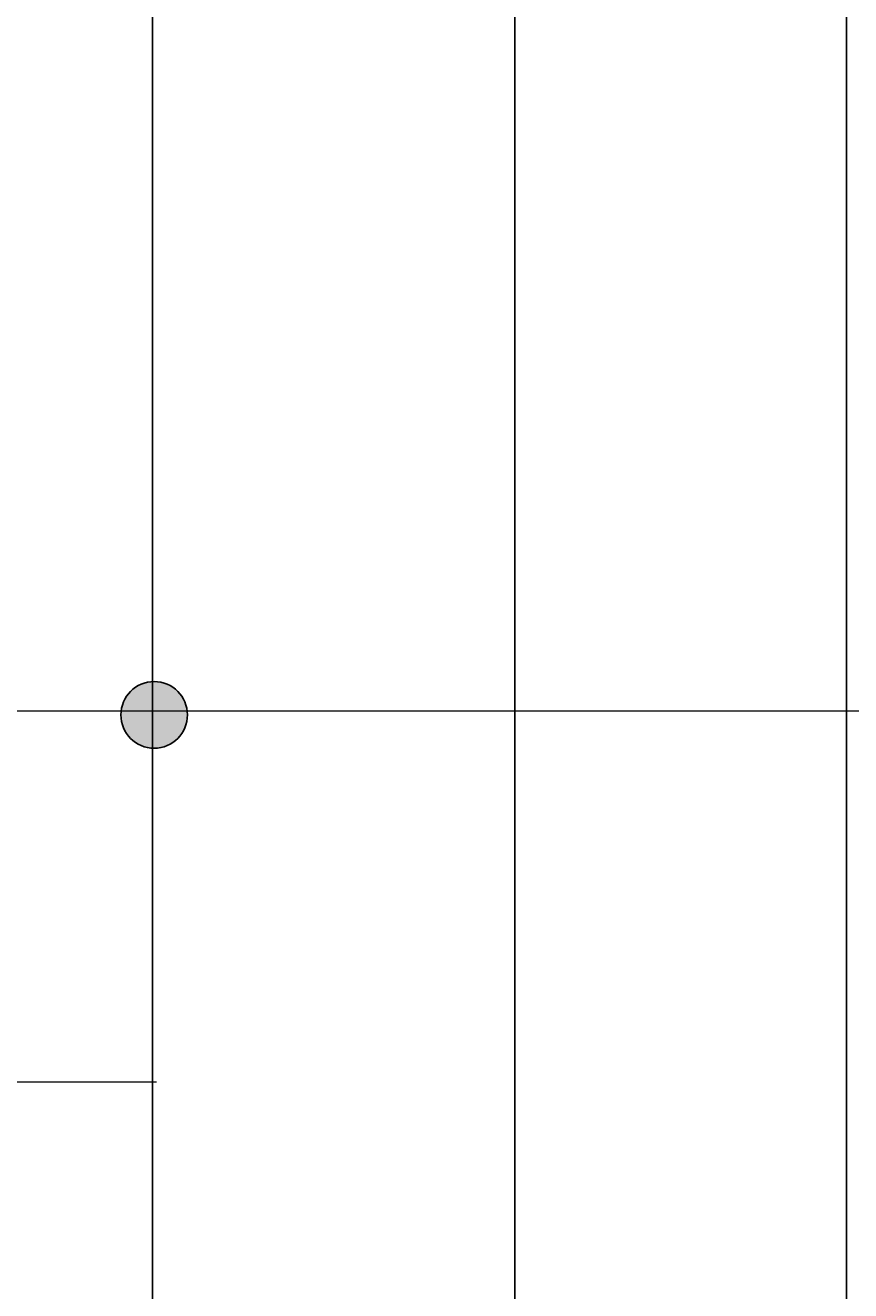
# Model space of a CAD drawing. Units: inches. Extents: x 738 to 1068, y 378 to 757.
# Tile 18 of 41: x 901 to 939, y 435 to 492. Entities that reach past the tile are written whole.
import ezdxf

# ---------------------------------------------------------------- set-up
doc = ezdxf.new("R2010")
doc.units = ezdxf.units.IN
doc.header["$MEASUREMENT"] = 0
for name, color, linetype, lineweight in [('A-ANNO-DIMS', 2, 'Continuous', 18), ('E-CONN', 7, 'Continuous', 25), ('E-CONN-PATT', 7, 'Continuous', 13), ('E-CTRL-WIRE', 7, 'Continuous', 18)]:
    doc.layers.add(name, color=color, linetype=linetype, lineweight=lineweight)
doc.styles.get("Standard").update_dxf_attribs({"font": 'arial.ttf'})
doc.dimstyles.get("Standard").update_dxf_attribs({"dimtxt": 0.18, "dimasz": 0.18, "dimexe": 0.18, "dimexo": 0.0625, "dimgap": 0.09, "dimtad": 0, "dimtih": 1, "dimtoh": 1, "dimdec": 4, "dimzin": 0, "dimdsep": 46, "dimtxsty": 'Standard', "dimcen": 0.09, "dimadec": 0, "dimazin": 0, "dimtfac": 1, "dimtdec": 4, "dimtofl": 0, "dimtmove": 0, "dimatfit": 3, "dimfxl": 1, "dimtolj": 1, "dimtzin": 0, "dimarcsym": 0})

# ---------------------------------------------------------------- blocks, each defined once
blk = doc.blocks.new('*D18')
at = {"layer": 'A-ANNO-DIMS', "color": 0, "lineweight": -2, "transparency": 16777216}
for p, q in [((901.525, 738.375), (1068.179, 738.375)), ((1067.999, 738.195), (1067.999, 569.167)), ((1067.999, 399.775), (1067.999, 568.803)), ((1023.842, 399.595), (1068.179, 399.595))]:
    blk.add_line(p, q, dxfattribs=at)
at = {"layer": 'A-ANNO-DIMS', "color": 0, "transparency": 16777216}
for points in [[(1067.969, 738.195), (1068.029, 738.195), (1067.999, 738.375)], [(1067.969, 399.775), (1068.029, 399.775), (1067.999, 399.595)]]:
    blk.add_solid(points, dxfattribs=at)
at = {"layer": 'Defpoints', "color": 0, "transparency": 16777216}
for p in [(901.462, 738.375), (1067.999, 738.375), (1023.779, 399.595)]:
    blk.add_point(p, dxfattribs=at)
at = {"layer": 'A-ANNO-DIMS', "color": 0, "transparency": 16777216, "insert": (1067.999, 568.985), "char_height": 0.18, "attachment_point": 5}
blk.add_mtext('\\A1;338.8', dxfattribs=at)
blk = doc.blocks.new('*D27')
at = {"layer": 'A-ANNO-DIMS', "color": 0, "lineweight": -2, "transparency": 16777216}
for p, q in [((883.457, 646.923), (883.457, 378.239)), ((923.511, 646.923), (923.511, 378.239)), ((883.637, 378.419), (903.086, 378.419)), ((923.331, 378.419), (903.882, 378.419))]:
    blk.add_line(p, q, dxfattribs=at)
at = {"layer": 'A-ANNO-DIMS', "color": 0, "transparency": 16777216}
for points in [[(883.637, 378.449), (883.637, 378.389), (883.457, 378.419)], [(923.331, 378.449), (923.331, 378.389), (923.511, 378.419)]]:
    blk.add_solid(points, dxfattribs=at)
at = {"layer": 'Defpoints', "color": 0, "transparency": 16777216}
for p in [(883.457, 646.985), (923.511, 646.985), (923.511, 378.419)]:
    blk.add_point(p, dxfattribs=at)
at = {"layer": 'A-ANNO-DIMS', "color": 0, "transparency": 16777216, "insert": (903.484, 378.419), "char_height": 0.18, "attachment_point": 5}
blk.add_mtext('\\A1;40.05', dxfattribs=at)
blk = doc.blocks.new('*D28')
at = {"layer": 'A-ANNO-DIMS', "color": 0, "lineweight": -2, "transparency": 16777216}
for p, q in [((923.511, 646.923), (923.511, 378.239)), ((969.439, 646.923), (969.439, 378.239)), ((923.691, 378.419), (946.078, 378.419)), ((969.259, 378.419), (946.872, 378.419))]:
    blk.add_line(p, q, dxfattribs=at)
at = {"layer": 'A-ANNO-DIMS', "color": 0, "transparency": 16777216}
for points in [[(923.691, 378.449), (923.691, 378.389), (923.511, 378.419)], [(969.259, 378.449), (969.259, 378.389), (969.439, 378.419)]]:
    blk.add_solid(points, dxfattribs=at)
at = {"layer": 'Defpoints', "color": 0, "transparency": 16777216}
for p in [(923.511, 646.985), (969.439, 646.985), (969.439, 378.419)]:
    blk.add_point(p, dxfattribs=at)
at = {"layer": 'A-ANNO-DIMS', "color": 0, "transparency": 16777216, "insert": (946.475, 378.419), "char_height": 0.18, "attachment_point": 5}
blk.add_mtext('\\A1;45.93', dxfattribs=at)
blk = doc.blocks.new('*D33')
at = {"layer": 'A-ANNO-DIMS', "color": 0, "lineweight": -2, "transparency": 16777216}
for p, q in [((836.324, 514.624), (836.324, 378.239)), ((907.171, 514.624), (907.171, 378.239)), ((836.504, 378.419), (871.354, 378.419)), ((906.991, 378.419), (872.141, 378.419))]:
    blk.add_line(p, q, dxfattribs=at)
at = {"layer": 'A-ANNO-DIMS', "color": 0, "transparency": 16777216}
for points in [[(836.504, 378.449), (836.504, 378.389), (836.324, 378.419)], [(906.991, 378.449), (906.991, 378.389), (907.171, 378.419)]]:
    blk.add_solid(points, dxfattribs=at)
at = {"layer": 'Defpoints', "color": 0, "transparency": 16777216}
for p in [(836.324, 514.687), (907.171, 514.687), (907.171, 378.419)]:
    blk.add_point(p, dxfattribs=at)
at = {"layer": 'A-ANNO-DIMS', "color": 0, "transparency": 16777216, "insert": (871.748, 378.419), "char_height": 0.18, "attachment_point": 5}
blk.add_mtext('\\A1;70.85', dxfattribs=at)
blk = doc.blocks.new('*D39')
at = {"layer": 'A-ANNO-DIMS', "color": 0, "lineweight": -2, "transparency": 16777216}
for p, q in [((887.04, 581.418), (887.04, 378.239)), ((938.455, 581.418), (938.455, 378.239)), ((887.22, 378.419), (912.371, 378.419)), ((938.275, 378.419), (913.124, 378.419))]:
    blk.add_line(p, q, dxfattribs=at)
at = {"layer": 'A-ANNO-DIMS', "color": 0, "transparency": 16777216}
for points in [[(887.22, 378.449), (887.22, 378.389), (887.04, 378.419)], [(938.275, 378.449), (938.275, 378.389), (938.455, 378.419)]]:
    blk.add_solid(points, dxfattribs=at)
at = {"layer": 'Defpoints', "color": 0, "transparency": 16777216}
for p in [(887.04, 581.481), (938.455, 581.481), (938.455, 378.419)]:
    blk.add_point(p, dxfattribs=at)
at = {"layer": 'A-ANNO-DIMS', "color": 0, "transparency": 16777216, "insert": (912.748, 378.419), "char_height": 0.18, "attachment_point": 5}
blk.add_mtext('\\A1;51.41', dxfattribs=at)

msp = doc.modelspace()

# ---------------------------------------------------------------- hatches: boundary and pattern name
at = {"layer": 'E-CONN-PATT'}
h = msp.add_hatch(color=256, dxfattribs=at)
h.dxf.hatch_style = 1
h.paths.add_polyline_path([(834.743, 461.3919), (837.7218, 461.3919, 0.8876841)])
h.paths.add_polyline_path([(837.7324, 461.214, 0.0297234), (837.7218, 461.3919), (834.743, 461.3919, 0.0297234), (834.7324, 461.214, 1)])
h.paths.add_polyline_path([(908.7522, 461.214, 0.0297234), (908.7416, 461.3919), (905.7628, 461.3919, 0.0297234), (905.7522, 461.214, 1)])
h.paths.add_polyline_path([(905.7628, 461.3919), (908.7416, 461.3919, 0.8876841)])

# ---------------------------------------------------------------- linework, layer by layer
at = {"layer": 'E-CONN'}
msp.add_lwpolyline([(905.7522, 461.214, 1), (908.7522, 461.214, 1)], format="xyb", close=True, dxfattribs=at)
at = {"layer": 'E-CTRL-WIRE'}
for p, q in [((885.9574, 461.3919), (966.9395, 461.3919)), ((907.1708, 459.6489), (907.1708, 444.6775)), ((877.3586, 444.6775), (907.3586, 444.6775))]:
    msp.add_line(p, q, dxfattribs=at)

# ---------------------------------------------------------------- dimensions: what is measured, and where the dimension line sits
at = {"layer": 'A-ANNO-DIMS'}
dim = msp.add_linear_dim(base=(1067.9992, 738.3751), p1=(1023.779, 399.5952), p2=(901.4622, 738.3751), angle=90, dimstyle='Standard', override={"dimdec": 1, "dimlfac": 1, "dimrnd": 0, "dimzin": 0, "dimdsep": 46, "dimlunit": 2}, dxfattribs=at)
dim.commit()
dim.dimension.update_dxf_attribs({"geometry": '*D18', "text_midpoint": (1067.9992, 568.9851)})
for base, p1, p2, picture, middle in [((923.5105, 378.4191), (883.4574, 646.9853), (923.5105, 646.9853), '*D27', (903.484, 378.4191)), ((969.4395, 378.4191), (923.5105, 646.9853), (969.4395, 646.9853), '*D28', (946.475, 378.4191)), ((938.455, 378.4191), (887.0404, 581.4808), (938.455, 581.4808), '*D39', (912.7477, 378.4191)), ((907.1708, 378.4191), (836.3244, 514.6866), (907.1708, 514.6866), '*D33', (871.7476, 378.4191))]:
    dim = msp.add_linear_dim(base=base, p1=p1, p2=p2, dimstyle='Standard', override={"dimdec": 2, "dimlfac": 1, "dimrnd": 0, "dimzin": 0, "dimdsep": 46, "dimlunit": 2}, dxfattribs=at)
    dim.commit()
    dim.dimension.update_dxf_attribs({"geometry": picture, "text_midpoint": middle})

doc.saveas('drawing.dxf')
